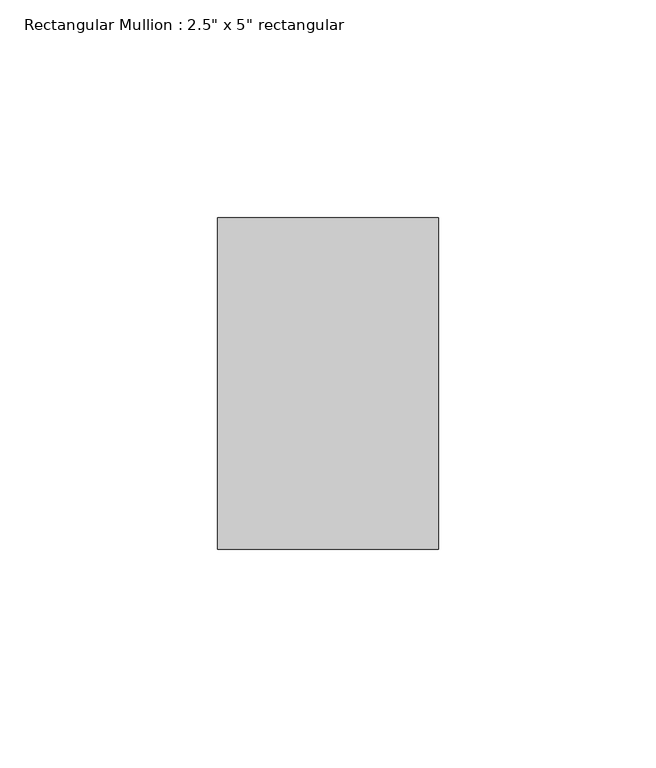
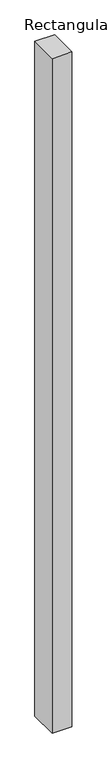
"""IFC4 building model written with IfcOpenShell, lengths in millimetres: member geometry."""

from ifc_helpers import new_model, si_unit, frame, origin, place, context, project, spatial, polyline, outline, extrude, source, transform, mapped, element, save


def member_86f0261c(model_context):
    return source(origin(), model_context, "Body", "SweptSolid", [
        extrude(outline(polyline([(0.0, 38.1), (0.0, -38.1), (-50.8, -38.1), (-50.8, 38.1), (0.0, 38.1)])), frame((0.0, 0.0, -1828.8), z_axis=(0.0, 0.0, 1.0), x_axis=(1.0, 0.0, 0.0)), (0.0, 0.0, 1.0), 1828.8),
    ])


if __name__ == "__main__":
    model = new_model("IFC4")
    model_context = context("Model", 3, world=origin())
    ifc_project = project(units=[si_unit("LENGTHUNIT", "METRE", prefix="MILLI")], contexts=[model_context])
    site = spatial("IfcSite", under=ifc_project)
    building = spatial("IfcBuilding", under=site)
    placement = place(None, origin())
    member_shape = member_86f0261c(model_context)
    element("IfcMember", 1, ObjectType="Rectangular Mullion : 2.5\" x 5\" rectangular", at=placement, inside=building, context=model_context, shape_type="MappedRepresentation", body=[
        mapped(member_shape, transform((0.0, 0.0, 0.0), x_axis=(1.0, 0.0, 0.0), y_axis=(0.0, 1.0, 0.0), z_axis=(0.0, 0.0, 1.0))),
    ])
    save(model, "model.ifc")

# Revit data of these elements
# Type "Rectangular Mullion : 2.5\" x 5\" rectangular"
#   built-in parameter 1007304 = 0.25 (stored number, unit not read)
#   built-in parameter 1007301 = 0.0833333 (stored number, unit not read)
#   built-in parameter 1007300 = 0.0833333 (stored number, unit not read)
# Element 1 (IfcMember, "Rectangular Mullion : 2.5\" x 5\" rectangular")
#   Materials on its faces: "Aluminum"
# Materials
#   "Aluminum": class "Metal", colour RGB 244 245 246, transparency 0, Description = "Aluminum 6061", Cost = 0
